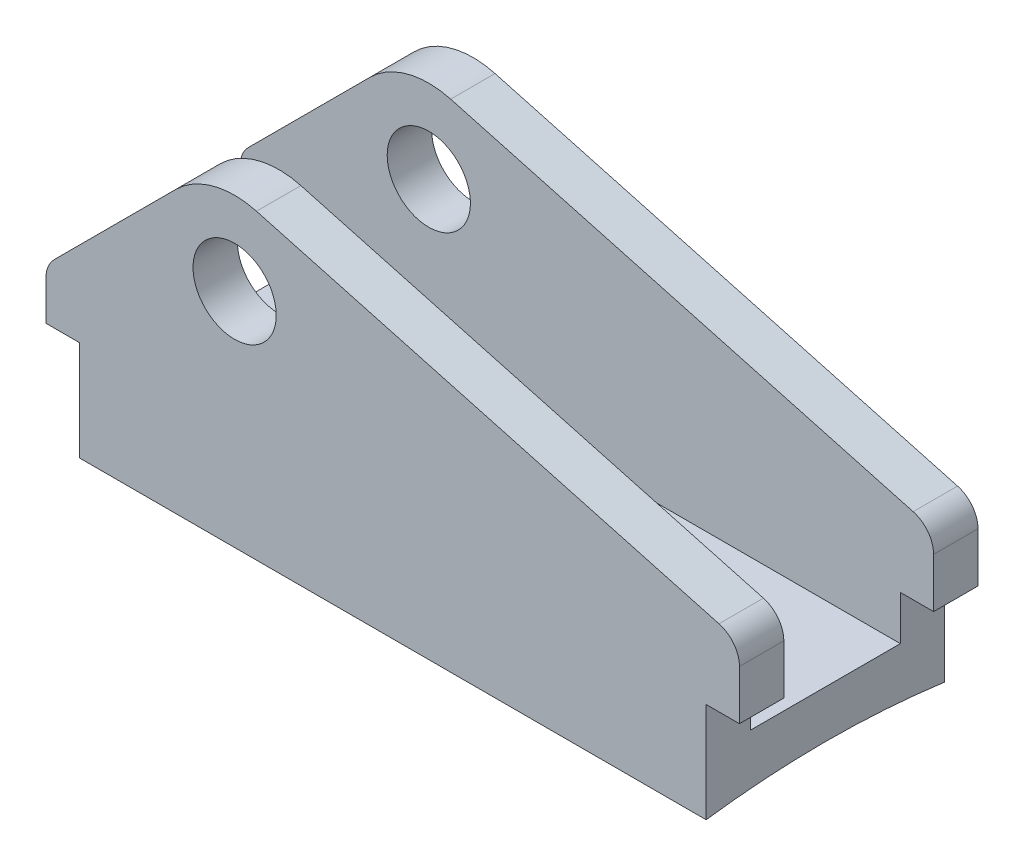
ISO-10303-21;
HEADER;
FILE_DESCRIPTION(('STEP AP214'),'2;1');
FILE_NAME('part.step','',(''),(''),'','','');
FILE_SCHEMA(('AUTOMOTIVE_DESIGN { 1 0 10303 214 1 1 1 1 }'));
ENDSEC;
DATA;
#1=APPLICATION_CONTEXT('core data for automotive mechanical design processes');
#2=APPLICATION_PROTOCOL_DEFINITION('international standard','automotive_design',2000,#1);
#3=PRODUCT_CONTEXT('',#1,'mechanical');
#4=PRODUCT('Part','Part','',(#3));
#5=PRODUCT_RELATED_PRODUCT_CATEGORY('part','',(#4));
#6=PRODUCT_DEFINITION_FORMATION('','',#4);
#7=PRODUCT_DEFINITION_CONTEXT('part definition',#1,'design');
#8=PRODUCT_DEFINITION('design','',#6,#7);
#9=PRODUCT_DEFINITION_SHAPE('','',#8);
#10=(LENGTH_UNIT() NAMED_UNIT(*) SI_UNIT(.MILLI.,.METRE.));
#11=(NAMED_UNIT(*) PLANE_ANGLE_UNIT() SI_UNIT($,.RADIAN.));
#12=(NAMED_UNIT(*) SI_UNIT($,.STERADIAN.) SOLID_ANGLE_UNIT());
#13=UNCERTAINTY_MEASURE_WITH_UNIT(LENGTH_MEASURE(1.E-05),#10,'distance_accuracy_value','');
#14=(GEOMETRIC_REPRESENTATION_CONTEXT(3) GLOBAL_UNCERTAINTY_ASSIGNED_CONTEXT((#13)) GLOBAL_UNIT_ASSIGNED_CONTEXT((#10,
#11,#12)) REPRESENTATION_CONTEXT('',''));
#15=CARTESIAN_POINT('',(0.,0.,0.));
#16=DIRECTION('',(0.,0.,1.));
#17=DIRECTION('',(1.,0.,0.));
#18=AXIS2_PLACEMENT_3D('',#15,#16,#17);
#19=CARTESIAN_POINT('',(-29.,-14.8578643762692,21.5));
#20=DIRECTION('',(0.,0.,-1.));
#21=DIRECTION('',(-1.,0.,0.));
#22=AXIS2_PLACEMENT_3D('',#19,#20,#21);
#23=CYLINDRICAL_SURFACE('',#22,5.);
#24=CARTESIAN_POINT('',(-29.,-14.8578643762692,-13.5));
#25=DIRECTION('',(0.,0.,-1.));
#26=DIRECTION('',(-1.,0.,0.));
#27=AXIS2_PLACEMENT_3D('',#24,#25,#26);
#28=CIRCLE('',#27,5.);
#29=CARTESIAN_POINT('',(-32.5355339059327,-11.3223304703364,-13.5));
#30=VERTEX_POINT('',#29);
#31=CARTESIAN_POINT('',(-34.,-14.8578643762692,-13.5));
#32=VERTEX_POINT('',#31);
#33=EDGE_CURVE('E289',#30,#32,#28,.F.);
#34=ORIENTED_EDGE('',*,*,#33,.F.);
#35=DIRECTION('',(0.,0.,-1.));
#36=VECTOR('',#35,1.);
#37=CARTESIAN_POINT('',(-32.5355339059327,-11.3223304703364,21.5));
#38=LINE('',#37,#36);
#39=CARTESIAN_POINT('',(-32.5355339059327,-11.3223304703364,-21.5));
#40=VERTEX_POINT('',#39);
#41=EDGE_CURVE('E107',#30,#40,#38,.T.);
#42=ORIENTED_EDGE('',*,*,#41,.T.);
#43=CARTESIAN_POINT('',(-29.,-14.8578643762692,-21.5));
#44=DIRECTION('',(0.,0.,1.));
#45=DIRECTION('',(1.,0.,0.));
#46=AXIS2_PLACEMENT_3D('',#43,#44,#45);
#47=CIRCLE('',#46,5.);
#48=CARTESIAN_POINT('',(-34.,-14.8578643762692,-21.5));
#49=VERTEX_POINT('',#48);
#50=EDGE_CURVE('E175',#49,#40,#47,.F.);
#51=ORIENTED_EDGE('',*,*,#50,.F.);
#52=DIRECTION('',(0.,0.,-1.));
#53=VECTOR('',#52,1.);
#54=CARTESIAN_POINT('',(-34.,-14.8578643762692,21.5));
#55=LINE('',#54,#53);
#56=EDGE_CURVE('E242',#32,#49,#55,.T.);
#57=ORIENTED_EDGE('',*,*,#56,.F.);
#58=EDGE_LOOP('',(#34,#42,#51,#57));
#59=FACE_BOUND('',#58,.T.);
#60=ADVANCED_FACE('F41',(#59),#23,.T.);
#61=CARTESIAN_POINT('',(-34.,0.,21.5));
#62=DIRECTION('',(-1.,0.,0.));
#63=DIRECTION('',(0.,-1.,0.));
#64=AXIS2_PLACEMENT_3D('',#61,#62,#63);
#65=PLANE('',#64);
#66=DIRECTION('',(0.,-1.,0.));
#67=VECTOR('',#66,1.);
#68=CARTESIAN_POINT('',(-34.,0.,-13.5));
#69=LINE('',#68,#67);
#70=CARTESIAN_POINT('',(-34.,-22.,-13.5));
#71=VERTEX_POINT('',#70);
#72=EDGE_CURVE('E288',#32,#71,#69,.T.);
#73=ORIENTED_EDGE('',*,*,#72,.F.);
#74=ORIENTED_EDGE('',*,*,#56,.T.);
#75=DIRECTION('',(0.,1.,0.));
#76=VECTOR('',#75,1.);
#77=CARTESIAN_POINT('',(-34.,0.,-21.5));
#78=LINE('',#77,#76);
#79=CARTESIAN_POINT('',(-34.,-22.,-21.5));
#80=VERTEX_POINT('',#79);
#81=EDGE_CURVE('E180',#80,#49,#78,.T.);
#82=ORIENTED_EDGE('',*,*,#81,.F.);
#83=DIRECTION('',(0.,0.,-1.));
#84=VECTOR('',#83,1.);
#85=CARTESIAN_POINT('',(-34.,-22.,21.5));
#86=LINE('',#85,#84);
#87=EDGE_CURVE('E236',#71,#80,#86,.T.);
#88=ORIENTED_EDGE('',*,*,#87,.F.);
#89=EDGE_LOOP('',(#73,#74,#82,#88));
#90=FACE_BOUND('',#89,.T.);
#91=ADVANCED_FACE('F462',(#90),#65,.T.);
#92=CARTESIAN_POINT('',(0.,-22.,21.5));
#93=DIRECTION('',(0.,-1.,0.));
#94=DIRECTION('',(0.,0.,-1.));
#95=AXIS2_PLACEMENT_3D('',#92,#93,#94);
#96=PLANE('',#95);
#97=DIRECTION('',(1.,0.,0.));
#98=VECTOR('',#97,1.);
#99=CARTESIAN_POINT('',(0.,-22.,-13.5));
#100=LINE('',#99,#98);
#101=CARTESIAN_POINT('',(-28.,-22.,-13.5));
#102=VERTEX_POINT('',#101);
#103=EDGE_CURVE('E295',#71,#102,#100,.T.);
#104=ORIENTED_EDGE('',*,*,#103,.F.);
#105=ORIENTED_EDGE('',*,*,#87,.T.);
#106=DIRECTION('',(-1.,0.,0.));
#107=VECTOR('',#106,1.);
#108=CARTESIAN_POINT('',(0.,-22.,-21.5));
#109=LINE('',#108,#107);
#110=CARTESIAN_POINT('',(-28.,-22.,-21.5));
#111=VERTEX_POINT('',#110);
#112=EDGE_CURVE('E185',#111,#80,#109,.T.);
#113=ORIENTED_EDGE('',*,*,#112,.F.);
#114=DIRECTION('',(0.,0.,-1.));
#115=VECTOR('',#114,1.);
#116=CARTESIAN_POINT('',(-28.,-22.,21.5));
#117=LINE('',#116,#115);
#118=EDGE_CURVE('E233',#102,#111,#117,.T.);
#119=ORIENTED_EDGE('',*,*,#118,.F.);
#120=EDGE_LOOP('',(#104,#105,#113,#119));
#121=FACE_BOUND('',#120,.T.);
#122=ADVANCED_FACE('F404',(#121),#96,.T.);
#123=CARTESIAN_POINT('',(0.,-22.,21.5));
#124=DIRECTION('',(0.,-1.,0.));
#125=DIRECTION('',(0.,0.,-1.));
#126=AXIS2_PLACEMENT_3D('',#123,#124,#125);
#127=PLANE('',#126);
#128=DIRECTION('',(1.,0.,0.));
#129=VECTOR('',#128,1.);
#130=CARTESIAN_POINT('',(0.,-22.,-13.5));
#131=LINE('',#130,#129);
#132=CARTESIAN_POINT('',(85.,-22.,-13.5));
#133=VERTEX_POINT('',#132);
#134=CARTESIAN_POINT('',(91.,-22.,-13.5));
#135=VERTEX_POINT('',#134);
#136=EDGE_CURVE('E278',#133,#135,#131,.T.);
#137=ORIENTED_EDGE('',*,*,#136,.F.);
#138=DIRECTION('',(0.,0.,-1.));
#139=VECTOR('',#138,1.);
#140=CARTESIAN_POINT('',(85.,-22.,21.5));
#141=LINE('',#140,#139);
#142=CARTESIAN_POINT('',(85.,-22.,-21.5));
#143=VERTEX_POINT('',#142);
#144=EDGE_CURVE('E230',#133,#143,#141,.T.);
#145=ORIENTED_EDGE('',*,*,#144,.T.);
#146=DIRECTION('',(-1.,0.,0.));
#147=VECTOR('',#146,1.);
#148=CARTESIAN_POINT('',(0.,-22.,-21.5));
#149=LINE('',#148,#147);
#150=CARTESIAN_POINT('',(91.,-22.,-21.5));
#151=VERTEX_POINT('',#150);
#152=EDGE_CURVE('E193',#151,#143,#149,.T.);
#153=ORIENTED_EDGE('',*,*,#152,.F.);
#154=DIRECTION('',(0.,0.,-1.));
#155=VECTOR('',#154,1.);
#156=CARTESIAN_POINT('',(91.,-22.,21.5));
#157=LINE('',#156,#155);
#158=EDGE_CURVE('E226',#135,#151,#157,.T.);
#159=ORIENTED_EDGE('',*,*,#158,.F.);
#160=EDGE_LOOP('',(#137,#145,#153,#159));
#161=FACE_BOUND('',#160,.T.);
#162=ADVANCED_FACE('F529',(#161),#127,.T.);
#163=CARTESIAN_POINT('',(91.,0.,21.5));
#164=DIRECTION('',(1.,0.,0.));
#165=DIRECTION('',(0.,0.,-1.));
#166=AXIS2_PLACEMENT_3D('',#163,#164,#165);
#167=PLANE('',#166);
#168=DIRECTION('',(0.,1.,0.));
#169=VECTOR('',#168,1.);
#170=CARTESIAN_POINT('',(91.,0.,-13.5));
#171=LINE('',#170,#169);
#172=CARTESIAN_POINT('',(91.,-13.0684036036208,-13.5));
#173=VERTEX_POINT('',#172);
#174=EDGE_CURVE('E280',#135,#173,#171,.T.);
#175=ORIENTED_EDGE('',*,*,#174,.F.);
#176=ORIENTED_EDGE('',*,*,#158,.T.);
#177=DIRECTION('',(0.,-1.,0.));
#178=VECTOR('',#177,1.);
#179=CARTESIAN_POINT('',(91.,0.,-21.5));
#180=LINE('',#179,#178);
#181=CARTESIAN_POINT('',(91.,-13.0684036036208,-21.5));
#182=VERTEX_POINT('',#181);
#183=EDGE_CURVE('E197',#182,#151,#180,.T.);
#184=ORIENTED_EDGE('',*,*,#183,.F.);
#185=DIRECTION('',(0.,0.,-1.));
#186=VECTOR('',#185,1.);
#187=CARTESIAN_POINT('',(91.,-13.0684036036208,21.5));
#188=LINE('',#187,#186);
#189=EDGE_CURVE('E225',#173,#182,#188,.T.);
#190=ORIENTED_EDGE('',*,*,#189,.F.);
#191=EDGE_LOOP('',(#175,#176,#184,#190));
#192=FACE_BOUND('',#191,.T.);
#193=ADVANCED_FACE('F538',(#192),#167,.T.);
#194=CARTESIAN_POINT('',(86.,-13.0684036036208,21.5));
#195=DIRECTION('',(0.,0.,-1.));
#196=DIRECTION('',(-1.,0.,0.));
#197=AXIS2_PLACEMENT_3D('',#194,#195,#196);
#198=CYLINDRICAL_SURFACE('',#197,5.);
#199=DIRECTION('',(0.,0.,-1.));
#200=VECTOR('',#199,1.);
#201=CARTESIAN_POINT('',(87.3144607815624,-8.24427748029702,21.5));
#202=LINE('',#201,#200);
#203=CARTESIAN_POINT('',(87.3144607815624,-8.24427748029702,-13.5));
#204=VERTEX_POINT('',#203);
#205=CARTESIAN_POINT('',(87.3144607815624,-8.24427748029702,-21.5));
#206=VERTEX_POINT('',#205);
#207=EDGE_CURVE('E151',#204,#206,#202,.T.);
#208=ORIENTED_EDGE('',*,*,#207,.F.);
#209=CARTESIAN_POINT('',(86.,-13.0684036036208,-13.5));
#210=DIRECTION('',(0.,0.,-1.));
#211=DIRECTION('',(-1.,0.,0.));
#212=AXIS2_PLACEMENT_3D('',#209,#210,#211);
#213=CIRCLE('',#212,5.);
#214=EDGE_CURVE('E273',#204,#173,#213,.T.);
#215=ORIENTED_EDGE('',*,*,#214,.T.);
#216=ORIENTED_EDGE('',*,*,#189,.T.);
#217=CARTESIAN_POINT('',(86.,-13.0684036036208,-21.5));
#218=DIRECTION('',(0.,0.,1.));
#219=DIRECTION('',(1.,0.,0.));
#220=AXIS2_PLACEMENT_3D('',#217,#218,#219);
#221=CIRCLE('',#220,5.);
#222=EDGE_CURVE('E199',#182,#206,#221,.T.);
#223=ORIENTED_EDGE('',*,*,#222,.T.);
#224=EDGE_LOOP('',(#208,#215,#216,#223));
#225=FACE_BOUND('',#224,.T.);
#226=ADVANCED_FACE('F550',(#225),#198,.T.);
#227=CARTESIAN_POINT('',(3.94338234468715,14.4723783699712,21.5));
#228=DIRECTION('',(0.262892156312476,0.964825224664745,0.));
#229=DIRECTION('',(-0.964825224664745,0.262892156312476,0.));
#230=AXIS2_PLACEMENT_3D('',#227,#228,#229);
#231=PLANE('',#230);
#232=DIRECTION('',(-0.964825224664745,0.262892156312476,0.));
#233=VECTOR('',#232,1.);
#234=CARTESIAN_POINT('',(3.94338234468715,14.4723783699712,-13.5));
#235=LINE('',#234,#233);
#236=CARTESIAN_POINT('',(3.94338234468715,14.4723783699712,-13.5));
#237=VERTEX_POINT('',#236);
#238=EDGE_CURVE('E271',#204,#237,#235,.T.);
#239=ORIENTED_EDGE('',*,*,#238,.F.);
#240=ORIENTED_EDGE('',*,*,#207,.T.);
#241=DIRECTION('',(0.964825224664745,-0.262892156312476,0.));
#242=VECTOR('',#241,1.);
#243=CARTESIAN_POINT('',(3.94338234468715,14.4723783699712,-21.5));
#244=LINE('',#243,#242);
#245=CARTESIAN_POINT('',(3.94338234468715,14.4723783699712,-21.5));
#246=VERTEX_POINT('',#245);
#247=EDGE_CURVE('E201',#246,#206,#244,.T.);
#248=ORIENTED_EDGE('',*,*,#247,.F.);
#249=DIRECTION('',(0.,0.,-1.));
#250=VECTOR('',#249,1.);
#251=CARTESIAN_POINT('',(3.94338234468715,14.4723783699712,21.5));
#252=LINE('',#251,#250);
#253=EDGE_CURVE('E155',#237,#246,#252,.T.);
#254=ORIENTED_EDGE('',*,*,#253,.F.);
#255=EDGE_LOOP('',(#239,#240,#248,#254));
#256=FACE_BOUND('',#255,.T.);
#257=ADVANCED_FACE('F556',(#256),#231,.T.);
#258=CARTESIAN_POINT('',(0.,0.,21.5));
#259=DIRECTION('',(0.,0.,-1.));
#260=DIRECTION('',(-1.,0.,0.));
#261=AXIS2_PLACEMENT_3D('',#258,#259,#260);
#262=CYLINDRICAL_SURFACE('',#261,15.);
#263=CARTESIAN_POINT('',(0.,0.,-13.5));
#264=DIRECTION('',(0.,0.,-1.));
#265=DIRECTION('',(-1.,0.,0.));
#266=AXIS2_PLACEMENT_3D('',#263,#264,#265);
#267=CIRCLE('',#266,15.);
#268=CARTESIAN_POINT('',(-10.6066017177982,10.6066017177982,-13.5));
#269=VERTEX_POINT('',#268);
#270=EDGE_CURVE('E254',#269,#237,#267,.T.);
#271=ORIENTED_EDGE('',*,*,#270,.T.);
#272=ORIENTED_EDGE('',*,*,#253,.T.);
#273=CARTESIAN_POINT('',(0.,0.,-21.5));
#274=DIRECTION('',(0.,0.,1.));
#275=DIRECTION('',(1.,0.,0.));
#276=AXIS2_PLACEMENT_3D('',#273,#274,#275);
#277=CIRCLE('',#276,15.);
#278=CARTESIAN_POINT('',(-10.6066017177982,10.6066017177982,-21.5));
#279=VERTEX_POINT('',#278);
#280=EDGE_CURVE('E206',#246,#279,#277,.T.);
#281=ORIENTED_EDGE('',*,*,#280,.T.);
#282=DIRECTION('',(0.,0.,-1.));
#283=VECTOR('',#282,1.);
#284=CARTESIAN_POINT('',(-10.6066017177982,10.6066017177982,21.5));
#285=LINE('',#284,#283);
#286=EDGE_CURVE('E217',#269,#279,#285,.T.);
#287=ORIENTED_EDGE('',*,*,#286,.F.);
#288=EDGE_LOOP('',(#271,#272,#281,#287));
#289=FACE_BOUND('',#288,.T.);
#290=ADVANCED_FACE('F477',(#289),#262,.T.);
#291=CARTESIAN_POINT('',(-10.6066017177982,10.6066017177982,21.5));
#292=DIRECTION('',(0.707106781186549,-0.707106781186546,0.));
#293=DIRECTION('',(0.707106781186546,0.707106781186549,0.));
#294=AXIS2_PLACEMENT_3D('',#291,#292,#293);
#295=PLANE('',#294);
#296=ORIENTED_EDGE('',*,*,#41,.F.);
#297=DIRECTION('',(0.707106781186546,0.707106781186549,0.));
#298=VECTOR('',#297,1.);
#299=CARTESIAN_POINT('',(-10.6066017177982,10.6066017177982,-13.5));
#300=LINE('',#299,#298);
#301=EDGE_CURVE('E247',#30,#269,#300,.T.);
#302=ORIENTED_EDGE('',*,*,#301,.T.);
#303=ORIENTED_EDGE('',*,*,#286,.T.);
#304=DIRECTION('',(-0.707106781186546,-0.707106781186549,0.));
#305=VECTOR('',#304,1.);
#306=CARTESIAN_POINT('',(-10.6066017177982,10.6066017177982,-21.5));
#307=LINE('',#306,#305);
#308=EDGE_CURVE('E207',#279,#40,#307,.T.);
#309=ORIENTED_EDGE('',*,*,#308,.T.);
#310=EDGE_LOOP('',(#296,#302,#303,#309));
#311=FACE_BOUND('',#310,.T.);
#312=ADVANCED_FACE('F471',(#311),#295,.F.);
#313=CARTESIAN_POINT('',(0.,0.,21.5));
#314=DIRECTION('',(0.,0.,-1.));
#315=DIRECTION('',(-1.,0.,0.));
#316=AXIS2_PLACEMENT_3D('',#313,#314,#315);
#317=CYLINDRICAL_SURFACE('',#316,7.5);
#318=CARTESIAN_POINT('',(0.,0.,-13.5));
#319=DIRECTION('',(0.,0.,-1.));
#320=DIRECTION('',(-1.,0.,0.));
#321=AXIS2_PLACEMENT_3D('',#318,#319,#320);
#322=CIRCLE('',#321,7.5);
#323=CARTESIAN_POINT('',(-7.5,0.,-13.5));
#324=VERTEX_POINT('',#323);
#325=EDGE_CURVE('E250',#324,#324,#322,.T.);
#326=ORIENTED_EDGE('',*,*,#325,.F.);
#327=EDGE_LOOP('',(#326));
#328=FACE_BOUND('',#327,.T.);
#329=CARTESIAN_POINT('',(0.,0.,-21.5));
#330=DIRECTION('',(0.,0.,1.));
#331=DIRECTION('',(1.,0.,0.));
#332=AXIS2_PLACEMENT_3D('',#329,#330,#331);
#333=CIRCLE('',#332,7.5);
#334=CARTESIAN_POINT('',(7.5,0.,-21.5));
#335=VERTEX_POINT('',#334);
#336=EDGE_CURVE('E211',#335,#335,#333,.T.);
#337=ORIENTED_EDGE('',*,*,#336,.F.);
#338=EDGE_LOOP('',(#337));
#339=FACE_BOUND('',#338,.T.);
#340=ADVANCED_FACE('F470',(#328,#339),#317,.F.);
#341=CARTESIAN_POINT('',(-29.,-14.8578643762692,13.5));
#342=DIRECTION('',(0.,0.,1.));
#343=DIRECTION('',(0.,-1.,0.));
#344=AXIS2_PLACEMENT_3D('',#341,#342,#343);
#345=CIRCLE('',#344,5.);
#346=CARTESIAN_POINT('',(-34.,-14.8578643762692,13.5));
#347=VERTEX_POINT('',#346);
#348=CARTESIAN_POINT('',(-32.5355339059327,-11.3223304703364,13.5));
#349=VERTEX_POINT('',#348);
#350=EDGE_CURVE('E57',#347,#349,#345,.F.);
#351=ORIENTED_EDGE('',*,*,#350,.F.);
#352=CARTESIAN_POINT('',(-34.,-14.8578643762692,21.5));
#353=VERTEX_POINT('',#352);
#354=EDGE_CURVE('E47',#353,#347,#55,.T.);
#355=ORIENTED_EDGE('',*,*,#354,.F.);
#356=CARTESIAN_POINT('',(-29.,-14.8578643762692,21.5));
#357=DIRECTION('',(0.,0.,1.));
#358=DIRECTION('',(1.,0.,0.));
#359=AXIS2_PLACEMENT_3D('',#356,#357,#358);
#360=CIRCLE('',#359,5.);
#361=CARTESIAN_POINT('',(-32.5355339059327,-11.3223304703364,21.5));
#362=VERTEX_POINT('',#361);
#363=EDGE_CURVE('E212',#353,#362,#360,.F.);
#364=ORIENTED_EDGE('',*,*,#363,.T.);
#365=EDGE_CURVE('E214',#362,#349,#38,.T.);
#366=ORIENTED_EDGE('',*,*,#365,.T.);
#367=EDGE_LOOP('',(#351,#355,#364,#366));
#368=FACE_BOUND('',#367,.T.);
#369=ADVANCED_FACE('F43',(#368),#23,.T.);
#370=DIRECTION('',(0.,1.,0.));
#371=VECTOR('',#370,1.);
#372=CARTESIAN_POINT('',(-34.,0.,13.5));
#373=LINE('',#372,#371);
#374=CARTESIAN_POINT('',(-34.,-22.,13.5));
#375=VERTEX_POINT('',#374);
#376=EDGE_CURVE('E264',#375,#347,#373,.T.);
#377=ORIENTED_EDGE('',*,*,#376,.F.);
#378=CARTESIAN_POINT('',(-34.,-22.,21.5));
#379=VERTEX_POINT('',#378);
#380=EDGE_CURVE('E239',#379,#375,#86,.T.);
#381=ORIENTED_EDGE('',*,*,#380,.F.);
#382=DIRECTION('',(0.,1.,0.));
#383=VECTOR('',#382,1.);
#384=CARTESIAN_POINT('',(-34.,0.,21.5));
#385=LINE('',#384,#383);
#386=EDGE_CURVE('E304',#379,#353,#385,.T.);
#387=ORIENTED_EDGE('',*,*,#386,.T.);
#388=ORIENTED_EDGE('',*,*,#354,.T.);
#389=EDGE_LOOP('',(#377,#381,#387,#388));
#390=FACE_BOUND('',#389,.T.);
#391=ADVANCED_FACE('F353',(#390),#65,.T.);
#392=DIRECTION('',(-1.,0.,0.));
#393=VECTOR('',#392,1.);
#394=CARTESIAN_POINT('',(0.,-22.,13.5));
#395=LINE('',#394,#393);
#396=CARTESIAN_POINT('',(-28.,-22.,13.5));
#397=VERTEX_POINT('',#396);
#398=EDGE_CURVE('E256',#397,#375,#395,.T.);
#399=ORIENTED_EDGE('',*,*,#398,.F.);
#400=CARTESIAN_POINT('',(-28.,-22.,21.5));
#401=VERTEX_POINT('',#400);
#402=EDGE_CURVE('E232',#401,#397,#117,.T.);
#403=ORIENTED_EDGE('',*,*,#402,.F.);
#404=DIRECTION('',(-1.,0.,0.));
#405=VECTOR('',#404,1.);
#406=CARTESIAN_POINT('',(0.,-22.,21.5));
#407=LINE('',#406,#405);
#408=EDGE_CURVE('E303',#401,#379,#407,.T.);
#409=ORIENTED_EDGE('',*,*,#408,.T.);
#410=ORIENTED_EDGE('',*,*,#380,.T.);
#411=EDGE_LOOP('',(#399,#403,#409,#410));
#412=FACE_BOUND('',#411,.T.);
#413=ADVANCED_FACE('F358',(#412),#96,.T.);
#414=CARTESIAN_POINT('',(-28.,0.,21.5));
#415=DIRECTION('',(-1.,0.,0.));
#416=DIRECTION('',(0.,0.,1.));
#417=AXIS2_PLACEMENT_3D('',#414,#415,#416);
#418=PLANE('',#417);
#419=DIRECTION('',(0.,-1.,0.));
#420=VECTOR('',#419,1.);
#421=CARTESIAN_POINT('',(-28.,0.,-13.5));
#422=LINE('',#421,#420);
#423=CARTESIAN_POINT('',(-28.,-30.,-13.5));
#424=VERTEX_POINT('',#423);
#425=EDGE_CURVE('E293',#102,#424,#422,.T.);
#426=ORIENTED_EDGE('',*,*,#425,.F.);
#427=ORIENTED_EDGE('',*,*,#118,.T.);
#428=DIRECTION('',(0.,1.,0.));
#429=VECTOR('',#428,1.);
#430=CARTESIAN_POINT('',(-28.,0.,-21.5));
#431=LINE('',#430,#429);
#432=CARTESIAN_POINT('',(-28.,-40.,-21.5));
#433=VERTEX_POINT('',#432);
#434=EDGE_CURVE('E183',#433,#111,#431,.T.);
#435=ORIENTED_EDGE('',*,*,#434,.F.);
#436=CARTESIAN_POINT('',(-28.,-198.548888359395,0.));
#437=DIRECTION('',(-1.,0.,0.));
#438=DIRECTION('',(0.,0.,1.));
#439=AXIS2_PLACEMENT_3D('',#436,#437,#438);
#440=CIRCLE('',#439,160.);
#441=CARTESIAN_POINT('',(-28.,-40.,21.5));
#442=VERTEX_POINT('',#441);
#443=EDGE_CURVE('E246',#442,#433,#440,.T.);
#444=ORIENTED_EDGE('',*,*,#443,.F.);
#445=DIRECTION('',(0.,1.,0.));
#446=VECTOR('',#445,1.);
#447=CARTESIAN_POINT('',(-28.,0.,21.5));
#448=LINE('',#447,#446);
#449=EDGE_CURVE('E307',#442,#401,#448,.T.);
#450=ORIENTED_EDGE('',*,*,#449,.T.);
#451=ORIENTED_EDGE('',*,*,#402,.T.);
#452=DIRECTION('',(0.,1.,0.));
#453=VECTOR('',#452,1.);
#454=CARTESIAN_POINT('',(-28.,0.,13.5));
#455=LINE('',#454,#453);
#456=CARTESIAN_POINT('',(-28.,-30.,13.5));
#457=VERTEX_POINT('',#456);
#458=EDGE_CURVE('E253',#457,#397,#455,.T.);
#459=ORIENTED_EDGE('',*,*,#458,.F.);
#460=DIRECTION('',(0.,0.,1.));
#461=VECTOR('',#460,1.);
#462=CARTESIAN_POINT('',(-28.,-30.,21.5));
#463=LINE('',#462,#461);
#464=EDGE_CURVE('E178',#424,#457,#463,.T.);
#465=ORIENTED_EDGE('',*,*,#464,.F.);
#466=EDGE_LOOP('',(#426,#427,#435,#444,#450,#451,#459,#465));
#467=FACE_BOUND('',#466,.T.);
#468=ADVANCED_FACE('F362',(#467),#418,.T.);
#469=CARTESIAN_POINT('',(85.,0.,21.5));
#470=DIRECTION('',(1.,0.,0.));
#471=DIRECTION('',(0.,0.,-1.));
#472=AXIS2_PLACEMENT_3D('',#469,#470,#471);
#473=PLANE('',#472);
#474=DIRECTION('',(0.,1.,0.));
#475=VECTOR('',#474,1.);
#476=CARTESIAN_POINT('',(85.,0.,-13.5));
#477=LINE('',#476,#475);
#478=CARTESIAN_POINT('',(85.,-30.,-13.5));
#479=VERTEX_POINT('',#478);
#480=EDGE_CURVE('E284',#479,#133,#477,.T.);
#481=ORIENTED_EDGE('',*,*,#480,.F.);
#482=DIRECTION('',(0.,0.,-1.));
#483=VECTOR('',#482,1.);
#484=CARTESIAN_POINT('',(85.,-30.,21.5));
#485=LINE('',#484,#483);
#486=CARTESIAN_POINT('',(85.,-30.,13.5));
#487=VERTEX_POINT('',#486);
#488=EDGE_CURVE('E11',#487,#479,#485,.T.);
#489=ORIENTED_EDGE('',*,*,#488,.F.);
#490=DIRECTION('',(0.,-1.,0.));
#491=VECTOR('',#490,1.);
#492=CARTESIAN_POINT('',(85.,0.,13.5));
#493=LINE('',#492,#491);
#494=CARTESIAN_POINT('',(85.,-22.,13.5));
#495=VERTEX_POINT('',#494);
#496=EDGE_CURVE('E337',#495,#487,#493,.T.);
#497=ORIENTED_EDGE('',*,*,#496,.F.);
#498=CARTESIAN_POINT('',(85.,-22.,21.5));
#499=VERTEX_POINT('',#498);
#500=EDGE_CURVE('E234',#499,#495,#141,.T.);
#501=ORIENTED_EDGE('',*,*,#500,.F.);
#502=DIRECTION('',(0.,-1.,0.));
#503=VECTOR('',#502,1.);
#504=CARTESIAN_POINT('',(85.,0.,21.5));
#505=LINE('',#504,#503);
#506=CARTESIAN_POINT('',(85.,-40.,21.5));
#507=VERTEX_POINT('',#506);
#508=EDGE_CURVE('E311',#499,#507,#505,.T.);
#509=ORIENTED_EDGE('',*,*,#508,.T.);
#510=CARTESIAN_POINT('',(85.,-198.548888359395,0.));
#511=DIRECTION('',(1.,0.,0.));
#512=DIRECTION('',(0.,0.,-1.));
#513=AXIS2_PLACEMENT_3D('',#510,#511,#512);
#514=CIRCLE('',#513,160.);
#515=CARTESIAN_POINT('',(85.,-40.,-21.5));
#516=VERTEX_POINT('',#515);
#517=EDGE_CURVE('E413',#516,#507,#514,.T.);
#518=ORIENTED_EDGE('',*,*,#517,.F.);
#519=DIRECTION('',(0.,-1.,0.));
#520=VECTOR('',#519,1.);
#521=CARTESIAN_POINT('',(85.,0.,-21.5));
#522=LINE('',#521,#520);
#523=EDGE_CURVE('E194',#143,#516,#522,.T.);
#524=ORIENTED_EDGE('',*,*,#523,.F.);
#525=ORIENTED_EDGE('',*,*,#144,.F.);
#526=EDGE_LOOP('',(#481,#489,#497,#501,#509,#518,#524,#525));
#527=FACE_BOUND('',#526,.T.);
#528=ADVANCED_FACE('F425',(#527),#473,.T.);
#529=DIRECTION('',(-1.,0.,0.));
#530=VECTOR('',#529,1.);
#531=CARTESIAN_POINT('',(0.,-22.,13.5));
#532=LINE('',#531,#530);
#533=CARTESIAN_POINT('',(91.,-22.,13.5));
#534=VERTEX_POINT('',#533);
#535=EDGE_CURVE('E332',#534,#495,#532,.T.);
#536=ORIENTED_EDGE('',*,*,#535,.F.);
#537=CARTESIAN_POINT('',(91.,-22.,21.5));
#538=VERTEX_POINT('',#537);
#539=EDGE_CURVE('E227',#538,#534,#157,.T.);
#540=ORIENTED_EDGE('',*,*,#539,.F.);
#541=DIRECTION('',(-1.,0.,0.));
#542=VECTOR('',#541,1.);
#543=CARTESIAN_POINT('',(0.,-22.,21.5));
#544=LINE('',#543,#542);
#545=EDGE_CURVE('E316',#538,#499,#544,.T.);
#546=ORIENTED_EDGE('',*,*,#545,.T.);
#547=ORIENTED_EDGE('',*,*,#500,.T.);
#548=EDGE_LOOP('',(#536,#540,#546,#547));
#549=FACE_BOUND('',#548,.T.);
#550=ADVANCED_FACE('F327',(#549),#127,.T.);
#551=DIRECTION('',(0.,-1.,0.));
#552=VECTOR('',#551,1.);
#553=CARTESIAN_POINT('',(91.,0.,13.5));
#554=LINE('',#553,#552);
#555=CARTESIAN_POINT('',(91.,-13.0684036036208,13.5));
#556=VERTEX_POINT('',#555);
#557=EDGE_CURVE('E339',#556,#534,#554,.T.);
#558=ORIENTED_EDGE('',*,*,#557,.F.);
#559=CARTESIAN_POINT('',(91.,-13.0684036036208,21.5));
#560=VERTEX_POINT('',#559);
#561=EDGE_CURVE('E224',#560,#556,#188,.T.);
#562=ORIENTED_EDGE('',*,*,#561,.F.);
#563=DIRECTION('',(0.,-1.,0.));
#564=VECTOR('',#563,1.);
#565=CARTESIAN_POINT('',(91.,0.,21.5));
#566=LINE('',#565,#564);
#567=EDGE_CURVE('E170',#560,#538,#566,.T.);
#568=ORIENTED_EDGE('',*,*,#567,.T.);
#569=ORIENTED_EDGE('',*,*,#539,.T.);
#570=EDGE_LOOP('',(#558,#562,#568,#569));
#571=FACE_BOUND('',#570,.T.);
#572=ADVANCED_FACE('F321',(#571),#167,.T.);
#573=ORIENTED_EDGE('',*,*,#561,.T.);
#574=CARTESIAN_POINT('',(86.,-13.0684036036208,13.5));
#575=DIRECTION('',(0.,0.,1.));
#576=DIRECTION('',(0.,-1.,0.));
#577=AXIS2_PLACEMENT_3D('',#574,#575,#576);
#578=CIRCLE('',#577,5.);
#579=CARTESIAN_POINT('',(87.3144607815624,-8.24427748029702,13.5));
#580=VERTEX_POINT('',#579);
#581=EDGE_CURVE('E344',#556,#580,#578,.T.);
#582=ORIENTED_EDGE('',*,*,#581,.T.);
#583=CARTESIAN_POINT('',(87.3144607815624,-8.24427748029702,21.5));
#584=VERTEX_POINT('',#583);
#585=EDGE_CURVE('E219',#584,#580,#202,.T.);
#586=ORIENTED_EDGE('',*,*,#585,.F.);
#587=CARTESIAN_POINT('',(86.,-13.0684036036208,21.5));
#588=DIRECTION('',(0.,0.,1.));
#589=DIRECTION('',(1.,0.,0.));
#590=AXIS2_PLACEMENT_3D('',#587,#588,#589);
#591=CIRCLE('',#590,5.);
#592=EDGE_CURVE('E163',#560,#584,#591,.T.);
#593=ORIENTED_EDGE('',*,*,#592,.F.);
#594=EDGE_LOOP('',(#573,#582,#586,#593));
#595=FACE_BOUND('',#594,.T.);
#596=ADVANCED_FACE('F445',(#595),#198,.T.);
#597=DIRECTION('',(0.964825224664745,-0.262892156312476,0.));
#598=VECTOR('',#597,1.);
#599=CARTESIAN_POINT('',(3.94338234468715,14.4723783699712,13.5));
#600=LINE('',#599,#598);
#601=CARTESIAN_POINT('',(3.94338234468715,14.4723783699712,13.5));
#602=VERTEX_POINT('',#601);
#603=EDGE_CURVE('E146',#602,#580,#600,.T.);
#604=ORIENTED_EDGE('',*,*,#603,.F.);
#605=CARTESIAN_POINT('',(3.94338234468715,14.4723783699712,21.5));
#606=VERTEX_POINT('',#605);
#607=EDGE_CURVE('E137',#606,#602,#252,.T.);
#608=ORIENTED_EDGE('',*,*,#607,.F.);
#609=DIRECTION('',(0.964825224664745,-0.262892156312476,0.));
#610=VECTOR('',#609,1.);
#611=CARTESIAN_POINT('',(3.94338234468715,14.4723783699712,21.5));
#612=LINE('',#611,#610);
#613=EDGE_CURVE('E144',#606,#584,#612,.T.);
#614=ORIENTED_EDGE('',*,*,#613,.T.);
#615=ORIENTED_EDGE('',*,*,#585,.T.);
#616=EDGE_LOOP('',(#604,#608,#614,#615));
#617=FACE_BOUND('',#616,.T.);
#618=ADVANCED_FACE('F142',(#617),#231,.T.);
#619=CARTESIAN_POINT('',(0.,0.,13.5));
#620=DIRECTION('',(0.,0.,1.));
#621=DIRECTION('',(0.,-1.,0.));
#622=AXIS2_PLACEMENT_3D('',#619,#620,#621);
#623=CIRCLE('',#622,15.);
#624=CARTESIAN_POINT('',(-10.6066017177982,10.6066017177982,13.5));
#625=VERTEX_POINT('',#624);
#626=EDGE_CURVE('E352',#602,#625,#623,.T.);
#627=ORIENTED_EDGE('',*,*,#626,.T.);
#628=CARTESIAN_POINT('',(-10.6066017177982,10.6066017177982,21.5));
#629=VERTEX_POINT('',#628);
#630=EDGE_CURVE('E158',#629,#625,#285,.T.);
#631=ORIENTED_EDGE('',*,*,#630,.F.);
#632=CARTESIAN_POINT('',(0.,0.,21.5));
#633=DIRECTION('',(0.,0.,1.));
#634=DIRECTION('',(1.,0.,0.));
#635=AXIS2_PLACEMENT_3D('',#632,#633,#634);
#636=CIRCLE('',#635,15.);
#637=EDGE_CURVE('E154',#606,#629,#636,.T.);
#638=ORIENTED_EDGE('',*,*,#637,.F.);
#639=ORIENTED_EDGE('',*,*,#607,.T.);
#640=EDGE_LOOP('',(#627,#631,#638,#639));
#641=FACE_BOUND('',#640,.T.);
#642=ADVANCED_FACE('F156',(#641),#262,.T.);
#643=ORIENTED_EDGE('',*,*,#630,.T.);
#644=DIRECTION('',(-0.707106781186546,-0.707106781186549,0.));
#645=VECTOR('',#644,1.);
#646=CARTESIAN_POINT('',(-10.6066017177982,10.6066017177982,13.5));
#647=LINE('',#646,#645);
#648=EDGE_CURVE('E249',#625,#349,#647,.T.);
#649=ORIENTED_EDGE('',*,*,#648,.T.);
#650=ORIENTED_EDGE('',*,*,#365,.F.);
#651=DIRECTION('',(-0.707106781186546,-0.707106781186549,0.));
#652=VECTOR('',#651,1.);
#653=CARTESIAN_POINT('',(-10.6066017177982,10.6066017177982,21.5));
#654=LINE('',#653,#652);
#655=EDGE_CURVE('E65',#629,#362,#654,.T.);
#656=ORIENTED_EDGE('',*,*,#655,.F.);
#657=EDGE_LOOP('',(#643,#649,#650,#656));
#658=FACE_BOUND('',#657,.T.);
#659=ADVANCED_FACE('F483',(#658),#295,.F.);
#660=CARTESIAN_POINT('',(0.,0.,13.5));
#661=DIRECTION('',(0.,0.,1.));
#662=DIRECTION('',(0.,-1.,0.));
#663=AXIS2_PLACEMENT_3D('',#660,#661,#662);
#664=CIRCLE('',#663,7.5);
#665=CARTESIAN_POINT('',(0.,-7.5,13.5));
#666=VERTEX_POINT('',#665);
#667=EDGE_CURVE('E243',#666,#666,#664,.T.);
#668=ORIENTED_EDGE('',*,*,#667,.F.);
#669=EDGE_LOOP('',(#668));
#670=FACE_BOUND('',#669,.T.);
#671=CARTESIAN_POINT('',(0.,0.,21.5));
#672=DIRECTION('',(0.,0.,1.));
#673=DIRECTION('',(1.,0.,0.));
#674=AXIS2_PLACEMENT_3D('',#671,#672,#673);
#675=CIRCLE('',#674,7.5);
#676=CARTESIAN_POINT('',(7.5,0.,21.5));
#677=VERTEX_POINT('',#676);
#678=EDGE_CURVE('E172',#677,#677,#675,.T.);
#679=ORIENTED_EDGE('',*,*,#678,.T.);
#680=EDGE_LOOP('',(#679));
#681=FACE_BOUND('',#680,.T.);
#682=ADVANCED_FACE('F478',(#670,#681),#317,.F.);
#683=CARTESIAN_POINT('',(0.,0.,21.5));
#684=DIRECTION('',(0.,0.,1.));
#685=DIRECTION('',(1.,0.,0.));
#686=AXIS2_PLACEMENT_3D('',#683,#684,#685);
#687=PLANE('',#686);
#688=ORIENTED_EDGE('',*,*,#363,.F.);
#689=ORIENTED_EDGE('',*,*,#386,.F.);
#690=ORIENTED_EDGE('',*,*,#408,.F.);
#691=ORIENTED_EDGE('',*,*,#449,.F.);
#692=DIRECTION('',(-1.,0.,0.));
#693=VECTOR('',#692,1.);
#694=CARTESIAN_POINT('',(0.,-40.,21.5));
#695=LINE('',#694,#693);
#696=EDGE_CURVE('E309',#507,#442,#695,.T.);
#697=ORIENTED_EDGE('',*,*,#696,.F.);
#698=ORIENTED_EDGE('',*,*,#508,.F.);
#699=ORIENTED_EDGE('',*,*,#545,.F.);
#700=ORIENTED_EDGE('',*,*,#567,.F.);
#701=ORIENTED_EDGE('',*,*,#592,.T.);
#702=ORIENTED_EDGE('',*,*,#613,.F.);
#703=ORIENTED_EDGE('',*,*,#637,.T.);
#704=ORIENTED_EDGE('',*,*,#655,.T.);
#705=EDGE_LOOP('',(#688,#689,#690,#691,#697,#698,#699,#700,#701,#702,#703,#704));
#706=FACE_BOUND('',#705,.T.);
#707=ORIENTED_EDGE('',*,*,#678,.F.);
#708=EDGE_LOOP('',(#707));
#709=FACE_BOUND('',#708,.T.);
#710=ADVANCED_FACE('F159',(#706,#709),#687,.T.);
#711=CARTESIAN_POINT('',(0.,0.,-21.5));
#712=DIRECTION('',(0.,0.,1.));
#713=DIRECTION('',(1.,0.,0.));
#714=AXIS2_PLACEMENT_3D('',#711,#712,#713);
#715=PLANE('',#714);
#716=ORIENTED_EDGE('',*,*,#50,.T.);
#717=ORIENTED_EDGE('',*,*,#308,.F.);
#718=ORIENTED_EDGE('',*,*,#280,.F.);
#719=ORIENTED_EDGE('',*,*,#247,.T.);
#720=ORIENTED_EDGE('',*,*,#222,.F.);
#721=ORIENTED_EDGE('',*,*,#183,.T.);
#722=ORIENTED_EDGE('',*,*,#152,.T.);
#723=ORIENTED_EDGE('',*,*,#523,.T.);
#724=DIRECTION('',(-1.,0.,0.));
#725=VECTOR('',#724,1.);
#726=CARTESIAN_POINT('',(0.,-40.,-21.5));
#727=LINE('',#726,#725);
#728=EDGE_CURVE('E189',#516,#433,#727,.T.);
#729=ORIENTED_EDGE('',*,*,#728,.T.);
#730=ORIENTED_EDGE('',*,*,#434,.T.);
#731=ORIENTED_EDGE('',*,*,#112,.T.);
#732=ORIENTED_EDGE('',*,*,#81,.T.);
#733=EDGE_LOOP('',(#716,#717,#718,#719,#720,#721,#722,#723,#729,#730,#731,#732));
#734=FACE_BOUND('',#733,.T.);
#735=ORIENTED_EDGE('',*,*,#336,.T.);
#736=EDGE_LOOP('',(#735));
#737=FACE_BOUND('',#736,.T.);
#738=ADVANCED_FACE('F407',(#734,#737),#715,.F.);
#739=CARTESIAN_POINT('',(-101.5,-198.548888359395,0.));
#740=DIRECTION('',(1.,0.,0.));
#741=DIRECTION('',(0.,0.,-1.));
#742=AXIS2_PLACEMENT_3D('',#739,#740,#741);
#743=CYLINDRICAL_SURFACE('',#742,160.);
#744=ORIENTED_EDGE('',*,*,#443,.T.);
#745=ORIENTED_EDGE('',*,*,#728,.F.);
#746=ORIENTED_EDGE('',*,*,#517,.T.);
#747=ORIENTED_EDGE('',*,*,#696,.T.);
#748=EDGE_LOOP('',(#744,#745,#746,#747));
#749=FACE_BOUND('',#748,.T.);
#750=ADVANCED_FACE('F450',(#749),#743,.F.);
#751=CARTESIAN_POINT('',(-101.5,-30.,-13.5));
#752=DIRECTION('',(0.,0.,-1.));
#753=DIRECTION('',(-1.,0.,0.));
#754=AXIS2_PLACEMENT_3D('',#751,#752,#753);
#755=PLANE('',#754);
#756=ORIENTED_EDGE('',*,*,#425,.T.);
#757=DIRECTION('',(1.,0.,0.));
#758=VECTOR('',#757,1.);
#759=CARTESIAN_POINT('',(-101.5,-30.,-13.5));
#760=LINE('',#759,#758);
#761=EDGE_CURVE('E431',#424,#479,#760,.T.);
#762=ORIENTED_EDGE('',*,*,#761,.T.);
#763=ORIENTED_EDGE('',*,*,#480,.T.);
#764=ORIENTED_EDGE('',*,*,#136,.T.);
#765=ORIENTED_EDGE('',*,*,#174,.T.);
#766=ORIENTED_EDGE('',*,*,#214,.F.);
#767=ORIENTED_EDGE('',*,*,#238,.T.);
#768=ORIENTED_EDGE('',*,*,#270,.F.);
#769=ORIENTED_EDGE('',*,*,#301,.F.);
#770=ORIENTED_EDGE('',*,*,#33,.T.);
#771=ORIENTED_EDGE('',*,*,#72,.T.);
#772=ORIENTED_EDGE('',*,*,#103,.T.);
#773=EDGE_LOOP('',(#756,#762,#763,#764,#765,#766,#767,#768,#769,#770,#771,#772));
#774=FACE_BOUND('',#773,.T.);
#775=ORIENTED_EDGE('',*,*,#325,.T.);
#776=EDGE_LOOP('',(#775));
#777=FACE_BOUND('',#776,.T.);
#778=ADVANCED_FACE('F399',(#774,#777),#755,.F.);
#779=CARTESIAN_POINT('',(-101.5,-30.,13.5));
#780=DIRECTION('',(0.,-1.,0.));
#781=DIRECTION('',(0.,0.,-1.));
#782=AXIS2_PLACEMENT_3D('',#779,#780,#781);
#783=PLANE('',#782);
#784=ORIENTED_EDGE('',*,*,#464,.T.);
#785=DIRECTION('',(1.,0.,0.));
#786=VECTOR('',#785,1.);
#787=CARTESIAN_POINT('',(-101.5,-30.,13.5));
#788=LINE('',#787,#786);
#789=EDGE_CURVE('E430',#457,#487,#788,.T.);
#790=ORIENTED_EDGE('',*,*,#789,.T.);
#791=ORIENTED_EDGE('',*,*,#488,.T.);
#792=ORIENTED_EDGE('',*,*,#761,.F.);
#793=EDGE_LOOP('',(#784,#790,#791,#792));
#794=FACE_BOUND('',#793,.T.);
#795=ADVANCED_FACE('F429',(#794),#783,.F.);
#796=CARTESIAN_POINT('',(-101.5,15.,13.5));
#797=DIRECTION('',(0.,0.,1.));
#798=DIRECTION('',(0.,-1.,0.));
#799=AXIS2_PLACEMENT_3D('',#796,#797,#798);
#800=PLANE('',#799);
#801=ORIENTED_EDGE('',*,*,#458,.T.);
#802=ORIENTED_EDGE('',*,*,#398,.T.);
#803=ORIENTED_EDGE('',*,*,#376,.T.);
#804=ORIENTED_EDGE('',*,*,#350,.T.);
#805=ORIENTED_EDGE('',*,*,#648,.F.);
#806=ORIENTED_EDGE('',*,*,#626,.F.);
#807=ORIENTED_EDGE('',*,*,#603,.T.);
#808=ORIENTED_EDGE('',*,*,#581,.F.);
#809=ORIENTED_EDGE('',*,*,#557,.T.);
#810=ORIENTED_EDGE('',*,*,#535,.T.);
#811=ORIENTED_EDGE('',*,*,#496,.T.);
#812=ORIENTED_EDGE('',*,*,#789,.F.);
#813=EDGE_LOOP('',(#801,#802,#803,#804,#805,#806,#807,#808,#809,#810,#811,#812));
#814=FACE_BOUND('',#813,.T.);
#815=ORIENTED_EDGE('',*,*,#667,.T.);
#816=EDGE_LOOP('',(#815));
#817=FACE_BOUND('',#816,.T.);
#818=ADVANCED_FACE('F347',(#814,#817),#800,.F.);
#819=CLOSED_SHELL('',(#60,#91,#122,#162,#193,#226,#257,#290,#312,#340,#369,#391,#413,#468,#528,
#550,#572,#596,#618,#642,#659,#682,#710,#738,#750,#778,#795,#818));
#820=MANIFOLD_SOLID_BREP('B2',#819);
#821=ADVANCED_BREP_SHAPE_REPRESENTATION('',(#18,#820),#14);
#822=SHAPE_DEFINITION_REPRESENTATION(#9,#821);
ENDSEC;
END-ISO-10303-21;
